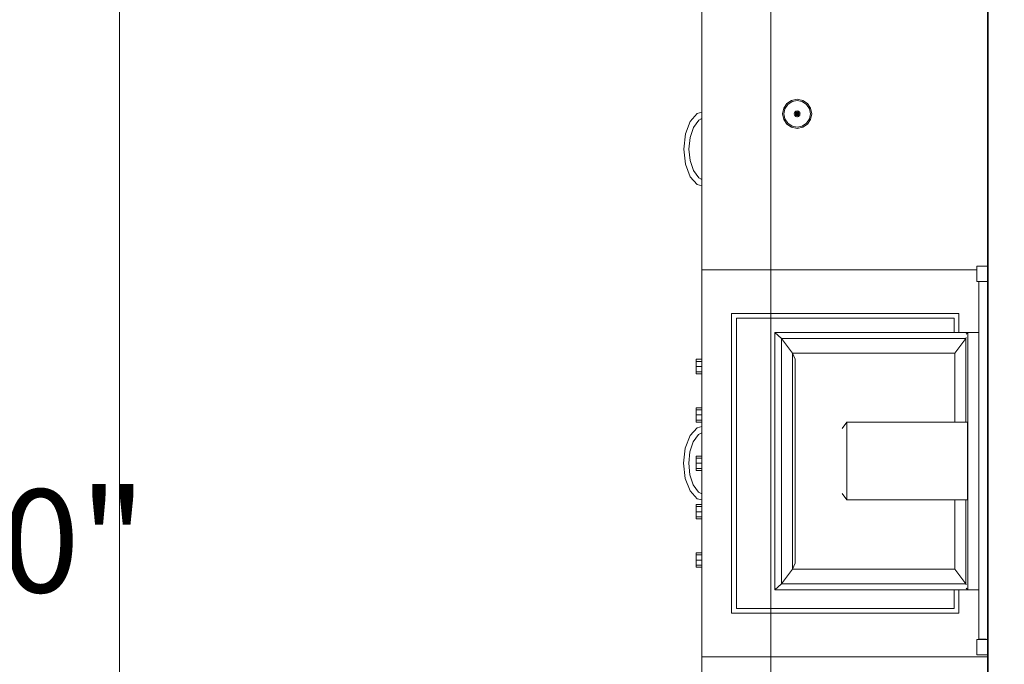
# Model space of a CAD drawing. Units: feet. Extents: x -297 to 770, y -228 to 625.
# Tile 10 of 14: x 680 to 734, y 158 to 194. Entities that reach past the tile are written whole.
import ezdxf

# ---------------------------------------------------------------- set-up
doc = ezdxf.new("R2010")
doc.units = ezdxf.units.FT
doc.header["$MEASUREMENT"] = 0
for name, color, linetype, lineweight in [('A-ANNO-DIMS', 2, 'Continuous', 18), ('A-AREA-IDEN', 7, 'Continuous', 25), ('A-EQPM', 8, 'Continuous', 13), ('A-FLOR-CASE', 8, 'Continuous', 18), ('A-WALL', 7, 'Continuous', 35), ('windows', 30, 'Continuous', 18)]:
    doc.layers.add(name, color=color, linetype=linetype, lineweight=lineweight)
doc.styles.add('Annotative', font='arial.ttf')
doc.styles.get("Standard").update_dxf_attribs({"font": 'arial.ttf'})
doc.dimstyles.get("Standard").update_dxf_attribs({"dimtxt": 3, "dimasz": 2, "dimexe": 0.18, "dimexo": 0.0625, "dimgap": 0.09, "dimtad": 1, "dimtoh": 1, "dimdec": 1, "dimzin": 0, "dimdsep": 46, "dimlunit": 3, "dimtxsty": 'Standard', "dimcen": 0, "dimclre": 256, "dimadec": 0, "dimazin": 0, "dimtfac": 1, "dimtdec": 1, "dimtofl": 0, "dimtmove": 0, "dimatfit": 3, "dimfxl": 1, "dimtolj": 1, "dimtzin": 0, "dimlwe": -1, "dimarcsym": 0})

# ---------------------------------------------------------------- blocks, each defined once
blk = doc.blocks.new('WIN-5FT')
for p, q in [((60, 6.5), (0, 6.5)), ((60, 2.5), (0, 2.5))]:
    blk.add_line(p, q)
blk.add_lwpolyline([(60, 0), (60, 9), (0, 9), (0, 0)], close=True)
blk = doc.blocks.new('*D68')
at = {"layer": 'A-ANNO-DIMS', "transparency": 16777216}
for p, q in [((685.155, 306.9), (685.155, -227.667)), ((721.155, 306.9), (721.155, -227.667))]:
    blk.add_line(p, q, dxfattribs=at)
at = {"layer": 'A-ANNO-DIMS', "color": 0, "lineweight": -2, "transparency": 16777216}
blk.add_line((687.155, -227.487), (719.155, -227.487), dxfattribs=at)
at = {"layer": 'A-ANNO-DIMS', "color": 0, "transparency": 16777216}
for points in [[(687.155, -227.154), (687.155, -227.821), (685.155, -227.487)], [(719.155, -227.154), (719.155, -227.821), (721.155, -227.487)]]:
    blk.add_solid(points, dxfattribs=at)
at = {"layer": 'Defpoints', "color": 0, "transparency": 16777216}
for p in [(685.155, 306.963), (721.155, 306.963), (721.155, -227.487)]:
    blk.add_point(p, dxfattribs=at)
at = {"layer": 'A-ANNO-DIMS', "color": 0, "transparency": 16777216, "insert": (703.155, -225.865), "char_height": 3, "attachment_point": 5}
blk.add_mtext('\\A1;36', dxfattribs=at)

msp = doc.modelspace()

# ---------------------------------------------------------------- linework, layer by layer
at = {"layer": 'A-EQPM'}
for p, q in [((722.306, 189.512), (722.045, 189.338)), ((722.331, 189.451), (722.092, 189.291)), ((722.613, 189.573), (722.306, 189.512)), ((722.613, 189.507), (722.331, 189.451)), ((722.921, 189.512), (722.613, 189.573)), ((722.895, 189.451), (722.613, 189.507)), ((723.134, 189.291), (722.895, 189.451)), ((723.182, 189.338), (722.921, 189.512)), ((721.871, 189.077), (721.81, 188.77)), ((722.045, 189.338), (721.871, 189.077)), ((721.933, 189.052), (721.877, 188.77)), ((722.092, 189.291), (721.933, 189.052)), ((722.442, 188.841), (722.613, 188.77)), ((722.482, 188.901), (722.613, 188.77)), ((722.542, 188.941), (722.613, 188.77)), ((722.613, 188.77), (722.613, 188.955)), ((722.613, 188.77), (722.684, 188.941)), ((722.613, 188.77), (722.745, 188.901)), ((722.613, 188.77), (722.785, 188.841)), ((723.294, 189.052), (723.134, 189.291)), ((723.356, 189.077), (723.182, 189.338)), ((723.35, 188.77), (723.294, 189.052)), ((723.417, 188.77), (723.356, 189.077)), ((721.81, 188.77), (721.871, 188.462)), ((721.871, 188.462), (722.045, 188.201)), ((721.877, 188.77), (721.933, 188.488)), ((722.092, 188.249), (721.933, 188.488)), ((722.428, 188.77), (722.613, 188.77)), ((722.613, 188.77), (722.442, 188.699)), ((722.613, 188.77), (722.482, 188.638)), ((722.613, 188.77), (722.542, 188.598)), ((722.613, 188.77), (722.799, 188.77)), ((722.785, 188.699), (722.613, 188.77)), ((722.613, 188.77), (722.745, 188.638)), ((722.684, 188.598), (722.613, 188.77)), ((722.613, 188.77), (722.613, 188.584)), ((723.134, 188.249), (723.294, 188.488)), ((723.182, 188.201), (723.356, 188.462)), ((723.35, 188.77), (723.294, 188.488)), ((723.356, 188.462), (723.417, 188.77)), ((722.045, 188.201), (722.306, 188.027)), ((722.331, 188.089), (722.092, 188.249)), ((722.306, 188.027), (722.613, 187.966)), ((722.613, 188.033), (722.331, 188.089)), ((722.895, 188.089), (722.613, 188.033)), ((722.613, 187.966), (722.921, 188.027)), ((723.134, 188.249), (722.895, 188.089)), ((722.921, 188.027), (723.182, 188.201)), ((732.648, 159.723), (732.648, 179.495)), ((718.987, 177.738), (731.554, 177.738)), ((718.987, 161.157), (718.987, 177.738)), ((719.255, 177.471), (731.286, 177.471)), ((719.255, 161.424), (719.255, 177.471)), ((731.286, 177.471), (731.286, 176.687)), ((731.554, 177.738), (731.554, 176.687)), ((732.037, 176.687), (721.383, 176.687)), ((721.383, 176.687), (729.48, 176.687)), ((721.383, 176.687), (721.745, 176.347)), ((721.383, 162.445), (721.383, 176.687)), ((721.745, 176.347), (731.928, 176.347)), ((722.354, 175.536), (721.745, 176.347)), ((721.745, 176.347), (721.745, 162.785)), ((731.928, 176.347), (731.32, 175.536)), ((731.928, 176.347), (731.956, 176.411)), ((731.928, 171.724), (731.928, 176.347)), ((731.956, 176.58), (732.037, 176.687)), ((732.037, 176.687), (732.037, 162.445)), ((732.639, 176.687), (732.037, 176.687)), ((722.354, 175.536), (722.503, 175.196)), ((731.32, 175.536), (722.354, 175.536)), ((722.354, 163.596), (722.354, 175.536)), ((731.32, 171.724), (731.32, 175.536)), ((722.503, 175.196), (722.503, 163.936)), ((725.366, 171.724), (725.099, 171.367)), ((732.032, 171.724), (725.366, 171.724)), ((725.366, 167.423), (725.366, 171.724)), ((732.032, 167.423), (732.032, 171.724)), ((725.099, 167.779), (725.366, 167.423)), ((725.366, 167.423), (732.032, 167.423)), ((731.32, 163.596), (731.32, 167.423)), ((731.928, 162.785), (731.928, 167.423)), ((722.503, 163.936), (722.354, 163.596)), ((721.745, 162.785), (722.354, 163.596)), ((722.354, 163.596), (731.32, 163.596)), ((731.32, 163.596), (731.928, 162.785)), ((721.745, 162.785), (721.383, 162.445)), ((731.928, 162.785), (721.745, 162.785)), ((731.956, 162.722), (731.928, 162.785)), ((721.383, 162.445), (732.078, 162.445)), ((731.286, 162.445), (731.286, 161.424)), ((731.554, 162.445), (731.554, 161.157)), ((732.037, 162.445), (731.956, 162.552)), ((732.037, 162.445), (732.639, 162.445)), ((731.554, 161.157), (718.987, 161.157)), ((731.286, 161.424), (719.255, 161.424))]:
    msp.add_line(p, q, dxfattribs=at)
at = {"layer": 'A-FLOR-CASE'}
for p, q in [((733.155, 113.516), (733.155, 233.463)), ((717.351, 180.136), (717.351, 205.581)), ((717.088, 188.784), (717.351, 188.851)), ((716.703, 188.348), (716.439, 187.656)), ((717.088, 188.784), (716.703, 188.348)), ((717.171, 188.413), (716.883, 188.015)), ((717.351, 188.505), (717.171, 188.413)), ((716.883, 188.015), (716.696, 187.459)), ((716.439, 187.656), (716.346, 186.821)), ((716.696, 187.459), (716.631, 186.821)), ((716.346, 186.821), (716.439, 185.986)), ((716.631, 186.821), (716.696, 186.183)), ((716.696, 186.183), (716.883, 185.628)), ((716.439, 185.986), (716.703, 185.294)), ((716.883, 185.628), (717.171, 185.229)), ((716.703, 185.294), (717.088, 184.858)), ((717.171, 185.229), (717.351, 185.137)), ((717.088, 184.858), (717.351, 184.791)), ((717.341, 180.145), (717.351, 180.145)), ((717.341, 158.75), (717.341, 180.145)), ((717.484, 180.136), (717.351, 180.136)), ((717.484, 180.136), (732.539, 180.136)), ((732.539, 180.343), (733.158, 180.343)), ((732.539, 179.495), (732.539, 180.343)), ((733.158, 179.495), (732.539, 179.495)), ((717.035, 175.198), (717.341, 175.198)), ((717.035, 174.395), (717.035, 175.198)), ((717.035, 175.08), (717.341, 175.08)), ((717.035, 174.796), (717.341, 174.796)), ((717.035, 174.513), (717.341, 174.513)), ((717.341, 174.395), (717.035, 174.395)), ((717.035, 172.523), (717.341, 172.523)), ((717.035, 171.721), (717.035, 172.523)), ((717.035, 172.406), (717.341, 172.406)), ((717.035, 172.122), (717.341, 172.122)), ((717.035, 171.838), (717.341, 171.838)), ((717.341, 171.721), (717.035, 171.721)), ((717.078, 171.413), (717.341, 171.48)), ((716.693, 170.978), (716.43, 170.285)), ((717.078, 171.413), (716.693, 170.978)), ((717.161, 171.042), (716.873, 170.644)), ((717.341, 171.134), (717.161, 171.042)), ((716.873, 170.644), (716.686, 170.088)), ((716.43, 170.285), (716.336, 169.45)), ((716.686, 170.088), (716.621, 169.45)), ((717.035, 169.849), (717.341, 169.849)), ((717.035, 169.046), (717.035, 169.849)), ((716.336, 169.45), (716.43, 168.615)), ((716.621, 169.45), (716.686, 168.812)), ((717.035, 169.731), (717.341, 169.731)), ((717.035, 169.448), (717.341, 169.448)), ((716.686, 168.812), (716.873, 168.257)), ((717.035, 169.164), (717.341, 169.164)), ((717.341, 169.046), (717.035, 169.046)), ((716.43, 168.615), (716.693, 167.923)), ((716.873, 168.257), (717.161, 167.858)), ((716.693, 167.923), (717.078, 167.487)), ((717.161, 167.858), (717.341, 167.767)), ((717.035, 167.174), (717.341, 167.174)), ((717.035, 166.372), (717.035, 167.174)), ((717.078, 167.487), (717.341, 167.42)), ((717.035, 167.057), (717.341, 167.057)), ((717.035, 166.773), (717.341, 166.773)), ((717.035, 166.489), (717.341, 166.489)), ((717.341, 166.372), (717.035, 166.372)), ((717.035, 164.5), (717.341, 164.5)), ((717.035, 163.698), (717.035, 164.5)), ((717.035, 164.382), (717.341, 164.382)), ((717.035, 164.099), (717.341, 164.099)), ((717.035, 163.815), (717.341, 163.815)), ((717.341, 163.698), (717.035, 163.698)), ((732.539, 159.702), (733.158, 159.702)), ((732.539, 158.854), (732.539, 159.702)), ((733.06, 159.723), (732.648, 159.723)), ((717.346, 158.75), (717.341, 158.75)), ((717.346, 158.757), (717.479, 158.757)), ((717.346, 145.385), (717.346, 158.757)), ((717.479, 158.757), (733.158, 158.757)), ((733.158, 158.854), (732.539, 158.854))]:
    msp.add_line(p, q, dxfattribs=at)
at = {"layer": 'A-WALL'}
msp.add_lwpolyline([(733.155, 113.463), (733.155, 233.463)], dxfattribs=at)

# ---------------------------------------------------------------- block references
at = {"layer": 'windows', "rotation": 90.00000000000003}
msp.add_blockref('WIN-5FT', (742.155, 143.463), dxfattribs=at)

# ---------------------------------------------------------------- texts
at = {"layer": 'A-AREA-IDEN', "style": 'Annotative'}
msp.add_text('11\'0"X10\'0"', height=5.69601, dxfattribs=at).set_placement((644.619, 162.309))

# ---------------------------------------------------------------- dimensions: what is measured, and where the dimension line sits
at = {"layer": 'A-ANNO-DIMS'}
dim = msp.add_linear_dim(base=(721.155, -227.487), p1=(685.155, 306.963), p2=(721.155, 306.963), dimstyle='Standard', override={"dimdec": 0, "dimlfac": 1, "dimrnd": 0, "dimzin": 0, "dimdsep": 46, "dimlunit": 2}, dxfattribs=at)
dim.commit()
dim.dimension.update_dxf_attribs({"geometry": '*D68', "text_midpoint": (703.155, -225.865)})

doc.saveas('drawing.dxf')
